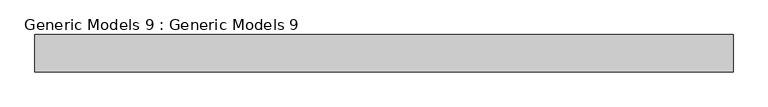
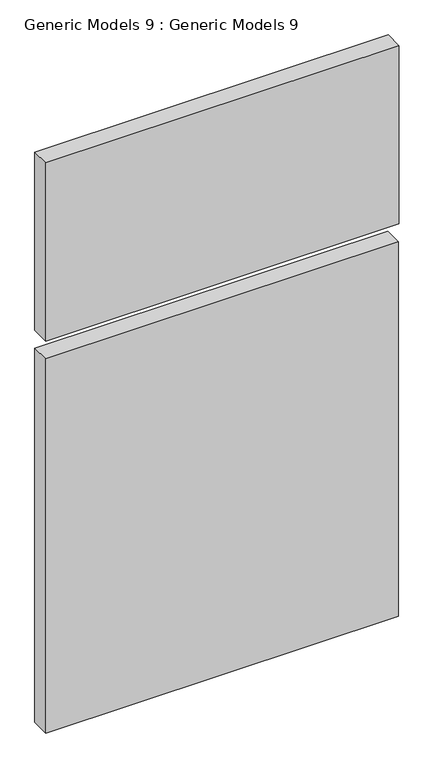
"""IFC4 building model written with IfcOpenShell, lengths in millimetres: proxy geometry, Generic Models 9 : Generic Models 9."""

from ifc_helpers import new_model, si_unit, frame, origin, place, context, project, spatial, polyline, outline, extrude, source, transform, mapped, element, save


def generic_models_9_generic_models_9_38eb4f00(model_context):
    return source(origin(), model_context, "Body", "SweptSolid", [
        extrude(outline(polyline([(-8003.2017815, -6684.6727897), (-10859.7771954, -6684.6727897), (-10859.7771954, -6532.2727897), (-8003.2017815, -6532.2727897), (-8003.2017815, -6684.6727897)])), frame((0.0, 0.0, 3200.4), z_axis=(0.0, 0.0, 1.0), x_axis=(1.0, 0.0, 0.0)), (0.0, 0.0, 1.0), 3200.4),
        extrude(outline(polyline([(-7999.1358708, -6684.6727897), (-10859.7771954, -6684.6727897), (-10859.7771954, -6532.2727897), (-7999.1358708, -6532.2727897), (-7999.1358708, -6684.6727897)])), frame((0.0, 0.0, 6553.2), z_axis=(0.0, 0.0, 1.0), x_axis=(1.0, 0.0, 0.0)), (0.0, 0.0, 1.0), 1524.0),
    ])


if __name__ == "__main__":
    model = new_model("IFC4")
    model_context = context("Model", 3, world=origin())
    ifc_project = project(units=[si_unit("LENGTHUNIT", "METRE", prefix="MILLI")], contexts=[model_context])
    site = spatial("IfcSite", under=ifc_project)
    building = spatial("IfcBuilding", under=site)
    placement = place(None, origin())
    generic_models_9_generic_models_9_shape = generic_models_9_generic_models_9_38eb4f00(model_context)
    element("IfcBuildingElementProxy", 1, Name="Generic Models 9 : Generic Models 9", ObjectType="Generic Models 9 : Generic Models 9", at=placement, inside=building, context=model_context, shape_type="MappedRepresentation", body=[
        mapped(generic_models_9_generic_models_9_shape, transform((0.0, 0.0, 0.0), x_axis=(1.0, 0.0, 0.0), y_axis=(0.0, 1.0, 0.0), z_axis=(0.0, 0.0, 1.0))),
    ])
    save(model, "model.ifc")
